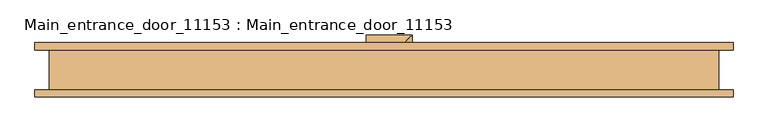
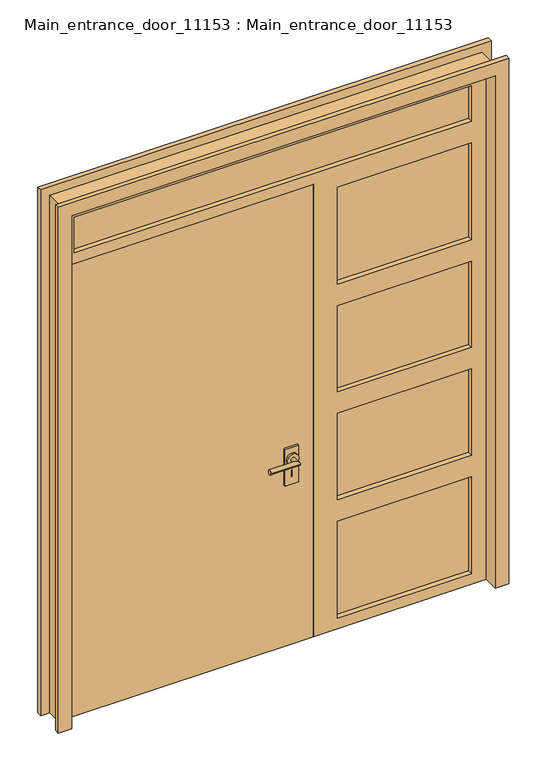
"""IFC4 building model written with IfcOpenShell, lengths in millimetres: door geometry, Main_entrance_door_11153 : Main_entrance_door_11153."""

from ifc_helpers import new_model, si_unit, point, frame, frame_2d, origin, origin_with_axes, place, context, project, spatial, polyline, circle_curve, ellipse_curve, trimmed, segment, composite_curve, outline, extrude, faceted_brep, source, transform, mapped, element, save
from ifc_brep_helpers import plane_surface, cylinder_surface, advanced_brep


def main_entrance_door_11153_main_entrance_door_11153_78fb3b47(model_context):
    return source(origin(), model_context, "Body", "SolidModel", [
        advanced_brep(
        [(60.0, 60.0, 870.0), (80.0, 60.0, 870.0), (80.0, 100.0, 870.0), (60.0, 80.0, 870.0), (-50.0, 80.0, 870.0), (-50.0, 100.0, 870.0)],
        [
            (0, 1, circle_curve(frame((70.0, 60.0, 870.0), z_axis=(0.0, -1.0, 0.0), x_axis=(1.0, 0.0, 0.0)), 10.0)),
            (1, 0, circle_curve(frame((70.0, 60.0, 870.0), z_axis=(0.0, -1.0, 0.0), x_axis=(1.0, 0.0, 0.0)), 10.0)),
            (1, 2),
            (2, 3, ellipse_curve(frame((70.0, 90.0, 870.0), z_axis=(0.7071067811865411, -0.7071067811865538, 0.0), x_axis=(-0.7071067811865538, -0.7071067811865412, 0.0)), 14.1421356, 10.0)),
            (3, 0),
            (3, 2, ellipse_curve(frame((70.0, 90.0, 870.0), z_axis=(0.7071067811865411, -0.7071067811865538, 0.0), x_axis=(-0.7071067811865538, -0.7071067811865412, 0.0)), 14.1421356, 10.0)),
            (4, 5, circle_curve(frame((-50.0, 90.0, 870.0), z_axis=(-1.0, 0.0, 0.0), x_axis=(0.0, 1.0, 0.0)), 10.0)),
            (5, 4, circle_curve(frame((-50.0, 90.0, 870.0), z_axis=(-1.0, 0.0, 0.0), x_axis=(0.0, 1.0, 0.0)), 10.0)),
            (2, 5),
            (4, 3),
        ],
        [
            plane_surface(frame((70.0, 60.0, 870.0), z_axis=(0.0, -1.0, 0.0), x_axis=(0.0, 0.0, 1.0))),
            cylinder_surface(frame((70.0, 60.0, 870.0), z_axis=(0.0, -1.0, 0.0), x_axis=(1.0, 0.0, 0.0)), 10.0),
            plane_surface(frame((-50.0, 90.0, 870.0), z_axis=(-1.0, 0.0, 0.0), x_axis=(0.0, 0.0, 1.0))),
            cylinder_surface(frame((70.0, 90.0, 870.0), z_axis=(1.0, 0.0, 0.0), x_axis=(0.0, 1.0, 0.0)), 10.0),
        ],
        [
            (0, [[1, 2]]),
            (1, [[3, 4, 5, -2]]),
            (1, [[-5, 6, -3, -1]]),
            (2, [[7, 8]]),
            (3, [[9, -7, 10, -4]]),
            (3, [[-10, -8, -9, -6]]),
        ],
    ),
        extrude(outline(polyline([(920.0, 100.0), (920.0, 40.0), (750.0, 40.0), (750.0, 100.0), (920.0, 100.0)]), holes=[polyline([(815.3510082, 71.5671262), (785.3510082, 71.5671262), (785.3510082, 68.4328738), (815.3510082, 68.4328738), (815.3510082, 71.5671262)])]), frame((0.0, 40.0, 0.0), z_axis=(0.0, 1.0, 0.0), x_axis=(0.0, 0.0, 1.0)), (0.0, 0.0, 1.0), 10.0),
        extrude(outline(composite_curve([segment(trimmed(circle_curve(frame_2d((870.0, 70.0)), 25.0), [point((870.0, 45.0))], [point((870.0, 95.0))], False, "CARTESIAN"), True, "CONTINUOUS"), segment(trimmed(circle_curve(frame_2d((870.0, 70.0)), 25.0), [point((870.0, 95.0))], [point((870.0, 45.0))], False, "CARTESIAN"), True, "CONTINUOUS")], self_intersect=False)), frame((0.0, 40.0, 0.0), z_axis=(0.0, 1.0, 0.0), x_axis=(0.0, 0.0, 1.0)), (0.0, 0.0, 1.0), 20.0),
        advanced_brep(
        [(60.0, -30.0, 870.0), (80.0, -30.0, 870.0), (60.0, -50.0, 870.0), (80.0, -70.0, 870.0), (-50.0, -50.0, 870.0), (-50.0, -70.0, 870.0)],
        [
            (0, 1, circle_curve(frame((70.0, -30.0, 870.0), z_axis=(0.0, 1.0, 0.0), x_axis=(1.0, 0.0, 0.0)), 10.0)),
            (1, 0, circle_curve(frame((70.0, -30.0, 870.0), z_axis=(0.0, 1.0, 0.0), x_axis=(1.0, 0.0, 0.0)), 10.0)),
            (0, 2),
            (2, 3, ellipse_curve(frame((70.0, -60.0, 870.0), z_axis=(0.7071067811865457, 0.7071067811865492, 0.0), x_axis=(-0.7071067811865492, 0.7071067811865458, 0.0)), 14.1421356, 10.0)),
            (3, 1),
            (3, 2, ellipse_curve(frame((70.0, -60.0, 870.0), z_axis=(0.7071067811865457, 0.7071067811865492, 0.0), x_axis=(-0.7071067811865492, 0.7071067811865458, 0.0)), 14.1421356, 10.0)),
            (4, 5, circle_curve(frame((-50.0, -60.0, 870.0), z_axis=(-1.0, 0.0, 0.0), x_axis=(0.0, -1.0, 0.0)), 10.0)),
            (5, 4, circle_curve(frame((-50.0, -60.0, 870.0), z_axis=(-1.0, 0.0, 0.0), x_axis=(0.0, -1.0, 0.0)), 10.0)),
            (2, 4),
            (5, 3),
        ],
        [
            plane_surface(frame((70.0, -30.0, 870.0), z_axis=(0.0, 1.0, 0.0), x_axis=(0.0, 0.0, 1.0))),
            cylinder_surface(frame((70.0, -30.0, 870.0), z_axis=(0.0, 1.0, 0.0), x_axis=(1.0, 0.0, 0.0)), 10.0),
            plane_surface(frame((-50.0, -60.0, 870.0), z_axis=(-1.0, 0.0, 0.0), x_axis=(0.0, 0.0, 1.0))),
            cylinder_surface(frame((70.0, -60.0, 870.0), z_axis=(1.0, 0.0, 0.0), x_axis=(0.0, -1.0, 0.0)), 10.0),
        ],
        [
            (0, [[1, 2]]),
            (1, [[-1, 3, 4, 5]]),
            (1, [[-2, -5, 6, -3]]),
            (2, [[7, 8]]),
            (3, [[-4, 9, -8, 10]]),
            (3, [[-6, -10, -7, -9]]),
        ],
    ),
        extrude(outline(polyline([(920.0, 100.0), (920.0, 40.0), (750.0, 40.0), (750.0, 100.0), (920.0, 100.0)]), holes=[polyline([(815.3510082, 71.5671262), (785.3510082, 71.5671262), (785.3510082, 68.4328738), (815.3510082, 68.4328738), (815.3510082, 71.5671262)])]), frame((0.0, -20.0, 0.0), z_axis=(0.0, 1.0, 0.0), x_axis=(0.0, 0.0, 1.0)), (0.0, 0.0, 1.0), 10.0),
        extrude(outline(composite_curve([segment(trimmed(circle_curve(frame_2d((870.0, 70.0)), 25.0), [point((870.0, 45.0))], [point((870.0, 95.0))], False, "CARTESIAN"), True, "CONTINUOUS"), segment(trimmed(circle_curve(frame_2d((870.0, 70.0)), 25.0), [point((870.0, 95.0))], [point((870.0, 45.0))], False, "CARTESIAN"), True, "CONTINUOUS")], self_intersect=False)), frame((0.0, -30.0, 0.0), z_axis=(0.0, 1.0, 0.0), x_axis=(0.0, 0.0, 1.0)), (0.0, 0.0, 1.0), 20.0),
        faceted_brep([(990.0, 57.15, 0.0), (950.0, 57.15, 0.0), (950.0, -57.15, 0.0), (990.0, -57.15, 0.0), (990.0, -77.15, 0.0), (930.0, -77.15, 0.0), (930.0, 40.0, 0.0), (915.0, 40.0, 0.0), (915.0, 55.0, 0.0), (930.0, 55.0, 0.0), (930.0, 77.15, 0.0), (990.0, 77.15, 0.0), (990.0, 57.15, 2440.0), (-990.0, 57.15, 2440.0), (-990.0, 57.15, 0.0), (-950.0, 57.15, 0.0), (-950.0, 57.15, 2400.0), (950.0, 57.15, 2400.0), (950.0, -57.15, 2400.0), (-950.0, -57.15, 2400.0), (-950.0, -57.15, 0.0), (-990.0, -57.15, 0.0), (-990.0, -57.15, 2440.0), (990.0, -57.15, 2440.0), (990.0, -77.15, 2440.0), (-990.0, -77.15, 2440.0), (-990.0, -77.15, 0.0), (-930.0, -77.15, 0.0), (-930.0, -77.15, 2380.0), (930.0, -77.15, 2380.0), (930.0, 40.0, 2380.0), (-930.0, 40.0, 2380.0), (-930.0, 40.0, 0.0), (-915.0, 40.0, 0.0), (-915.0, 40.0, 2365.0), (915.0, 40.0, 2365.0), (915.0, 55.0, 2365.0), (-915.0, 55.0, 2365.0), (-915.0, 55.0, 0.0), (-930.0, 55.0, 0.0), (-930.0, 55.0, 2380.0), (930.0, 55.0, 2380.0), (930.0, 77.15, 2380.0), (-930.0, 77.15, 2380.0), (-930.0, 77.15, 0.0), (-990.0, 77.15, 0.0), (-990.0, 77.15, 2440.0), (990.0, 77.15, 2440.0)], [[[0, 1, 2, 3, 4, 5, 6, 7, 8, 9, 10, 11]], [[1, 0, 12, 13, 14, 15, 16, 17]], [[2, 1, 17, 18]], [[3, 2, 18, 19, 20, 21, 22, 23]], [[4, 3, 23, 24]], [[5, 4, 24, 25, 26, 27, 28, 29]], [[6, 5, 29, 30]], [[7, 6, 30, 31, 32, 33, 34, 35]], [[8, 7, 35, 36]], [[9, 8, 36, 37, 38, 39, 40, 41]], [[10, 9, 41, 42]], [[11, 10, 42, 43, 44, 45, 46, 47]], [[0, 11, 47, 12]], [[14, 13, 46, 45]], [[15, 14, 45, 44, 39, 38, 33, 32, 27, 26, 21, 20]], [[16, 15, 20, 19]], [[22, 21, 26, 25]], [[28, 27, 32, 31]], [[34, 33, 38, 37]], [[40, 39, 44, 43]], [[13, 12, 47, 46]], [[17, 16, 19, 18]], [[23, 22, 25, 24]], [[29, 28, 31, 30]], [[35, 34, 37, 36]], [[41, 40, 43, 42]]]),
        faceted_brep([(225.0, 40.0, 0.0), (930.0, 40.0, 0.0), (930.0, -10.0, 0.0), (170.0, -10.0, 0.0), (170.0, 40.0, 0.0), (155.0, 40.0, 0.0), (155.0, 55.0, 0.0), (225.0, 55.0, 0.0), (225.0, 40.0, 2100.0), (930.0, 40.0, 2100.0), (865.0, 40.0, 500.0), (275.0, 40.0, 500.0), (275.0, 40.0, 50.0), (865.0, 40.0, 50.0), (865.0, 40.0, 1000.0), (275.0, 40.0, 1000.0), (275.0, 40.0, 600.0), (865.0, 40.0, 600.0), (865.0, 40.0, 1500.0), (275.0, 40.0, 1500.0), (275.0, 40.0, 1100.0), (865.0, 40.0, 1100.0), (865.0, 40.0, 2050.0), (275.0, 40.0, 2050.0), (275.0, 40.0, 1600.0), (865.0, 40.0, 1600.0), (930.0, 55.0, 2100.0), (930.0, 55.0, 2380.0), (930.0, -10.0, 2380.0), (-930.0, -10.0, 2380.0), (-930.0, -10.0, 2100.0), (170.0, -10.0, 2100.0), (275.0, -10.0, 500.0), (865.0, -10.0, 500.0), (865.0, -10.0, 50.0), (275.0, -10.0, 50.0), (275.0, -10.0, 1000.0), (865.0, -10.0, 1000.0), (865.0, -10.0, 600.0), (275.0, -10.0, 600.0), (-880.0, -10.0, 2315.0), (865.0, -10.0, 2315.0), (865.0, -10.0, 2150.0), (-880.0, -10.0, 2150.0), (275.0, -10.0, 1500.0), (865.0, -10.0, 1500.0), (865.0, -10.0, 1100.0), (275.0, -10.0, 1100.0), (275.0, -10.0, 2050.0), (865.0, -10.0, 2050.0), (865.0, -10.0, 1600.0), (275.0, -10.0, 1600.0), (170.0, 40.0, 2100.0), (155.0, 40.0, 2100.0), (155.0, 55.0, 2100.0), (-930.0, 55.0, 2100.0), (-930.0, 55.0, 2380.0), (225.0, 55.0, 2100.0), (865.0, 55.0, 2315.0), (-880.0, 55.0, 2315.0), (-880.0, 55.0, 2150.0), (865.0, 55.0, 2150.0)], [[[0, 1, 2, 3, 4, 5, 6, 7]], [[1, 0, 8, 9], [10, 11, 12, 13], [14, 15, 16, 17], [18, 19, 20, 21], [22, 23, 24, 25]], [[2, 1, 9, 26, 27, 28]], [[3, 2, 28, 29, 30, 31], [32, 33, 34, 35], [36, 37, 38, 39], [40, 41, 42, 43], [44, 45, 46, 47], [48, 49, 50, 51]], [[4, 3, 31, 52]], [[5, 4, 52, 53]], [[6, 5, 53, 54]], [[7, 6, 54, 55, 56, 27, 26, 57], [58, 59, 60, 61]], [[0, 7, 57, 8]], [[10, 33, 32, 11]], [[33, 10, 13, 34]], [[12, 35, 34, 13]], [[11, 32, 35, 12]], [[14, 37, 36, 15]], [[37, 14, 17, 38]], [[16, 39, 38, 17]], [[15, 36, 39, 16]], [[45, 18, 21, 46]], [[20, 47, 46, 21]], [[19, 44, 47, 20]], [[27, 56, 29, 28]], [[29, 56, 55, 30]], [[58, 41, 40, 59]], [[41, 58, 61, 42]], [[59, 40, 43, 60]], [[18, 45, 44, 19]], [[22, 49, 48, 23]], [[24, 51, 50, 25]], [[23, 48, 51, 24]], [[49, 22, 25, 50]], [[57, 26, 9, 8]], [[30, 55, 54, 53, 52, 31]], [[60, 43, 42, 61]]]),
        extrude(outline(polyline([(170.0, 40.0), (170.0, -10.0), (-930.0, -10.0), (-930.0, 40.0), (170.0, 40.0)])), origin_with_axes(), (0.0, 0.0, 1.0), 2100.0),
        extrude(outline(polyline([(-880.0, 12.0), (-880.0, 18.0), (865.0, 18.0), (865.0, 12.0), (-880.0, 12.0)])), frame((0.0, 0.0, 2150.0), z_axis=(0.0, 0.0, 1.0), x_axis=(1.0, 0.0, 0.0)), (0.0, 0.0, 1.0), 165.0),
        extrude(outline(polyline([(865.0, 18.0), (865.0, 12.0), (275.0, 12.0), (275.0, 18.0), (865.0, 18.0)])), frame((0.0, 0.0, 50.0), z_axis=(0.0, 0.0, 1.0), x_axis=(1.0, 0.0, 0.0)), (0.0, 0.0, 1.0), 450.0),
        extrude(outline(polyline([(865.0, 18.0), (865.0, 12.0), (275.0, 12.0), (275.0, 18.0), (865.0, 18.0)])), frame((0.0, 0.0, 600.0), z_axis=(0.0, 0.0, 1.0), x_axis=(1.0, 0.0, 0.0)), (0.0, 0.0, 1.0), 400.0),
        extrude(outline(polyline([(865.0, 18.0), (865.0, 12.0), (275.0, 12.0), (275.0, 18.0), (865.0, 18.0)])), frame((0.0, 0.0, 1600.0), z_axis=(0.0, 0.0, 1.0), x_axis=(1.0, 0.0, 0.0)), (0.0, 0.0, 1.0), 450.0),
        extrude(outline(polyline([(865.0, 18.0), (865.0, 12.0), (275.0, 12.0), (275.0, 18.0), (865.0, 18.0)])), frame((0.0, 0.0, 1100.0), z_axis=(0.0, 0.0, 1.0), x_axis=(1.0, 0.0, 0.0)), (0.0, 0.0, 1.0), 400.0),
    ])


if __name__ == "__main__":
    model = new_model("IFC4")
    model_context = context("Model", 3, world=origin())
    ifc_project = project(units=[si_unit("LENGTHUNIT", "METRE", prefix="MILLI")], contexts=[model_context])
    site = spatial("IfcSite", under=ifc_project)
    building = spatial("IfcBuilding", under=site)
    placement = place(None, origin())
    main_entrance_door_11153_main_entrance_door_11153_shape = main_entrance_door_11153_main_entrance_door_11153_78fb3b47(model_context)
    element("IfcDoor", 1, ObjectType="Main_entrance_door_11153 : Main_entrance_door_11153", at=placement, inside=building, context=model_context, shape_type="MappedRepresentation", body=[
        mapped(main_entrance_door_11153_main_entrance_door_11153_shape, transform((0.0, 0.0, 0.0), x_axis=(1.0, 0.0, 0.0), y_axis=(0.0, 1.0, 0.0), z_axis=(0.0, 0.0, 1.0))),
    ])
    save(model, "model.ifc")

# Revit data of these elements
# Type "Main_entrance_door_11153 : Main_entrance_door_11153"
#   Type Mark = "22"
#   Height = 7' - 10.48819"
#   Width = 6' - 2.80315"
#   Door Width = 3' - 7.30709"
#   Function = (empty or 0)
#   Wall Closure = (empty or 0)
# Element 1 (IfcDoor, "Main_entrance_door_11153 : Main_entrance_door_11153")
#   Materials on its faces: "Glass", "Default"
# Materials
#   "Glass": class "Glass", colour RGB 0 128 192, transparency 0.75, Description = "Soda Lime Glass", Cost = 0
#   "Default": colour RGB 127 127 127, transparency 0, Cost = 0
